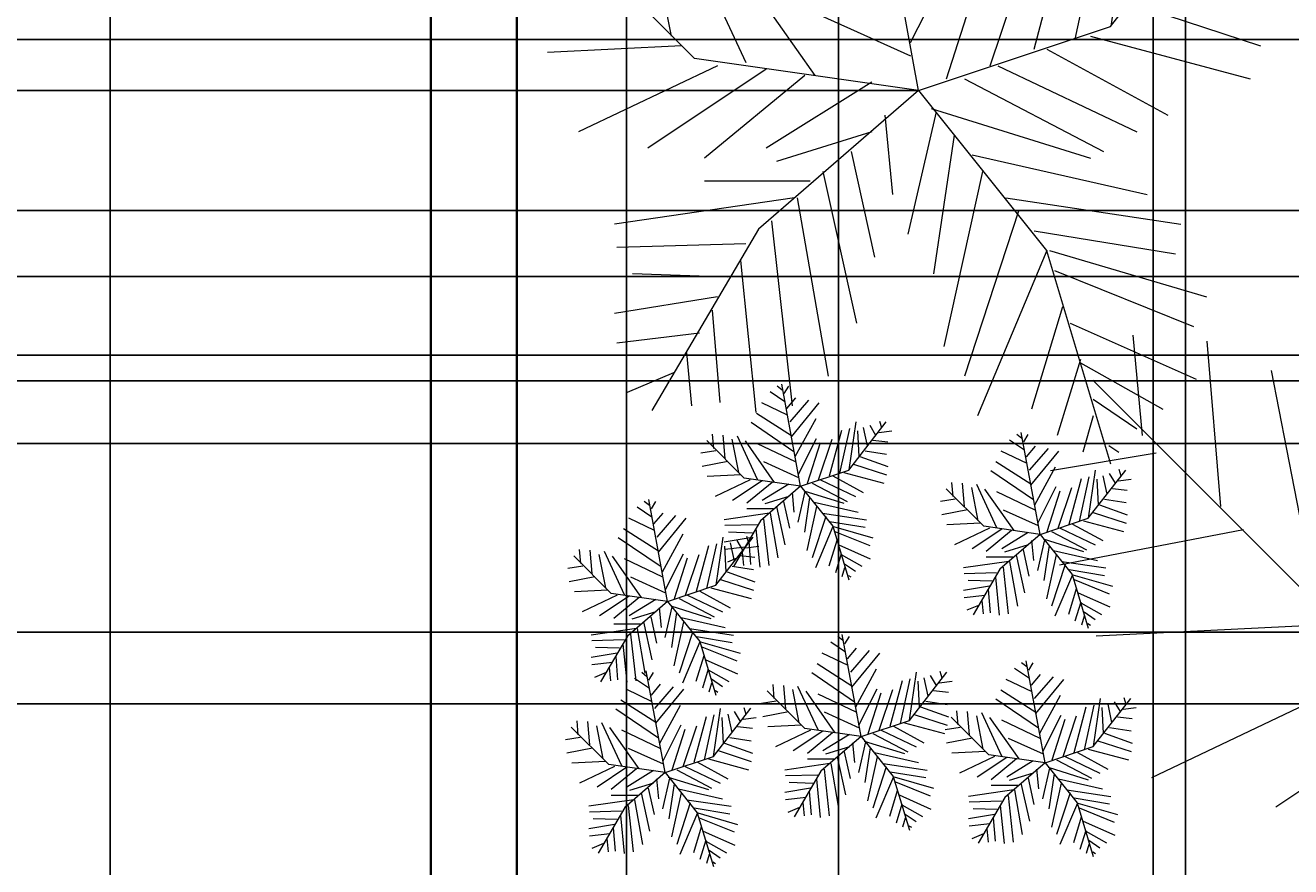
# Model space of a CAD drawing. Units: inches. Extents: x 818 to 1898, y 976 to 2364.
# Tile 59 of 96: x 950 to 1083, y 1958 to 2046. Entities that reach past the tile are written whole.
import ezdxf

# ---------------------------------------------------------------- set-up
doc = ezdxf.new("R2010")
doc.units = ezdxf.units.IN
doc.header["$LTSCALE"] = 5
doc.header["$MEASUREMENT"] = 0
for name, color, linetype, lineweight in [('A-ANNO-DIMS', 2, 'Continuous', 18), ('C-PROP', 7, 'Continuous', 35), ('L-PLNT-BEDS', 94, 'Continuous', 18)]:
    doc.layers.add(name, color=color, linetype=linetype, lineweight=lineweight)
doc.layers.add('L-PLNT', color=116, linetype='Continuous', lineweight=13, true_color=0x136734)
doc.styles.get("Standard").update_dxf_attribs({"font": 'arial.ttf'})
doc.dimstyles.get("Standard").update_dxf_attribs({"dimtxt": 0.18, "dimasz": 0.18, "dimexe": 0.18, "dimexo": 0.0625, "dimgap": 0.09, "dimtad": 0, "dimtih": 1, "dimtoh": 1, "dimdec": 4, "dimzin": 0, "dimdsep": 46, "dimtxsty": 'Standard', "dimcen": 0.09, "dimadec": 0, "dimazin": 0, "dimtfac": 1, "dimtdec": 4, "dimtofl": 0, "dimtmove": 0, "dimatfit": 3, "dimfxl": 1, "dimtolj": 1, "dimtzin": 0, "dimarcsym": 0})

# ---------------------------------------------------------------- blocks, each defined once
blk = doc.blocks.new('SHRUB-ACCENT')
for p, q in [((8.53, 19.84), (7.99, 20.28)), ((10.44, 9.82), (8.47, 20.47)), ((8.74, 19.5), (9.21, 20.28)), ((8.8, 18.63), (7.25, 19.67)), ((9.01, 17.93), (9.96, 19.06)), ((9.35, 16.54), (11.31, 18.8)), ((9.48, 15.07), (5.82, 17.41)), ((9.08, 17.24), (6.37, 18.54)), ((9.48, 14.98), (12.39, 18.54)), ((9.75, 13.42), (5.28, 16.46)), ((9.89, 12.9), (12.06, 16.89)), ((15.49, 11.5), (19.41, 16.55)), ((15.51, 11.51), (16.25, 16.54)), ((17, 15.94), (17.41, 14.03)), ((17.68, 16.2), (18.29, 15.16)), ((18.69, 16.63), (18.9, 15.94)), ((4.55, 10.66), (0.62, 14.58)), ((1.35, 13.77), (1.22, 15.24)), ((2.3, 15.16), (2.51, 12.72)), ((3.25, 14.72), (3.93, 11.25)), ((3.79, 15.07), (5.89, 10.55)), ((10.23, 11.07), (12.12, 14.81)), ((12.33, 10.47), (13.75, 14.72)), ((13.48, 10.9), (14.76, 15.68)), ((14.56, 11.16), (15.58, 15.85)), ((16.39, 15.59), (16.53, 12.9)), ((18.02, 14.63), (19.57, 14.46)), ((18.62, 15.42), (19.98, 15.59)), ((1.56, 13.51), (0, 13.25)), ((7.72, 10.21), (4.67, 14.55)), ((5.89, 14.29), (9.89, 12.38)), ((11.17, 10.12), (12.53, 14.37)), ((17.2, 13.51), (19.44, 13.16)), ((2.84, 12.38), (0.14, 11.86)), ((6.57, 12.38), (10.23, 10.73)), ((15.98, 12.12), (19.44, 10.99)), ((16.66, 12.9), (19.57, 11.86)), ((4.2, 10.99), (0.68, 10.81)), ((10.44, 9.82), (4.55, 10.66)), ((10.44, 9.82), (15.49, 11.5)), ((13.82, 10.9), (17, 9.16)), ((14.97, 11.25), (19.17, 10.12)), ((5.15, 10.47), (1.49, 8.73)), ((6.43, 10.38), (3.32, 8.3)), ((7.45, 10.21), (4.81, 8.04)), ((10.44, 9.82), (6.23, 6.17)), ((9.21, 10.03), (6.43, 8.3)), ((10.44, 9.82), (13.8, 5.61)), ((10.77, 9.34), (14.97, 8.04)), ((11.65, 10.12), (15.31, 8.21)), ((12.53, 10.47), (16.19, 8.73)), ((9.21, 8.73), (6.7, 7.95)), ((8.67, 8.21), (9.28, 5.43)), ((9.55, 9.16), (9.75, 7.08)), ((10.9, 9.25), (10.16, 6.04)), ((11.38, 8.64), (10.84, 5)), ((11.85, 8.12), (16.46, 7.08)), ((7.18, 6.99), (2.44, 6.3)), ((7.59, 7.43), (4.81, 7.43)), ((7.25, 6.99), (8.06, 2.31)), ((7.92, 7.69), (8.8, 3.69)), ((12.12, 7.69), (11.11, 3.09)), ((13.07, 6.65), (11.65, 2.31)), ((12.73, 6.99), (17.34, 6.3)), ((5.89, 5.78), (2.51, 5.69)), ((6.23, 6.17), (3.43, 1.4)), ((5.76, 5.34), (6.16, 1.35)), ((6.57, 6.39), (7.11, 1.52)), ((13.82, 5.6), (11.99, 1.26)), ((13.48, 6.13), (17.2, 5.52)), ((13.8, 5.61), (15.49, 0)), ((13.88, 5.6), (18.02, 4.39)), ((5.15, 4.39), (2.44, 3.95)), ((5.42, 4.91), (2.91, 5)), ((5.01, 4.04), (5.21, 1.61)), ((14.22, 4.13), (13.41, 1.44)), ((14.02, 5.08), (17.68, 3.61)), ((4.67, 3.43), (2.51, 3.17)), ((4.33, 2.91), (4.47, 1.52)), ((14.7, 2.74), (14.09, 0.74)), ((14.43, 3.69), (17.74, 2.22)), ((14.7, 2.65), (16.86, 1.44)), ((4, 2.39), (2.78, 1.87)), ((15.04, 1.7), (16.19, 0.92)), ((15.04, 1.26), (14.76, 0.31)), ((15.44, 0.48), (15.71, 0.31))]:
    blk.add_line(p, q)
blk = doc.blocks.new('PALM-BORDER')
for p, q in [((41.53, 39.05), (33.72, 81.45)), ((33.95, 78.95), (31.8, 80.68)), ((34.76, 77.57), (36.65, 80.68)), ((35.03, 74.11), (28.83, 78.26)), ((35.84, 71.35), (39.61, 75.84)), ((37.18, 65.82), (45, 74.8)), ((36.11, 68.59), (25.33, 73.77)), ((37.72, 59.6), (49.31, 73.77)), ((37.72, 59.95), (23.17, 69.28)), ((39.34, 51.31), (47.96, 67.2)), ((38.8, 53.39), (21.02, 65.48)), ((61.61, 45.75), (77.23, 65.83)), ((61.71, 45.79), (64.67, 65.82)), ((74.37, 66.17), (75.18, 63.4)), ((70.33, 64.44), (72.75, 60.3)), ((53.62, 43.37), (58.74, 62.37)), ((57.93, 44.41), (61.97, 63.06)), ((67.63, 63.4), (69.25, 55.81)), ((65.21, 62.02), (65.75, 51.31)), ((74.1, 61.33), (79.49, 62.02)), ((5.39, 54.77), (4.85, 60.64)), ((9.16, 60.3), (9.97, 50.62)), ((15.09, 59.95), (23.44, 41.99)), ((12.93, 58.57), (15.63, 44.75)), ((40.69, 44.06), (48.23, 58.91)), ((49.04, 41.64), (54.7, 58.57)), ((18.1, 42.4), (2.48, 58.02)), ((30.72, 40.61), (18.59, 57.88)), ((44.46, 40.26), (49.85, 57.19)), ((71.68, 58.22), (77.87, 57.53)), ((23.44, 56.84), (39.34, 49.24)), ((6.2, 53.73), (0, 52.7)), ((68.44, 53.73), (77.33, 52.35)), ((66.29, 51.31), (77.87, 47.17)), ((11.32, 49.24), (0.54, 47.17)), ((26.14, 49.24), (40.69, 42.68)), ((63.59, 48.21), (77.33, 43.71)), ((41.53, 39.05), (61.61, 45.75)), ((16.71, 43.71), (2.69, 43.02)), ((59.55, 44.75), (76.26, 40.26)), ((41.53, 39.05), (18.1, 42.4)), ((54.97, 43.37), (67.63, 36.46)), ((20.48, 41.64), (5.93, 34.73)), ((25.6, 41.3), (13.2, 33.01)), ((49.85, 41.64), (64.4, 34.73)), ((29.64, 40.61), (19.13, 31.97)), ((36.65, 39.91), (25.6, 33.01)), ((46.35, 40.26), (60.9, 32.66)), ((41.53, 39.05), (24.79, 24.55)), ((41.53, 39.05), (54.92, 22.32)), ((42.84, 37.15), (59.55, 31.97)), ((37.99, 36.46), (38.8, 28.17)), ((43.38, 36.81), (40.42, 24.02)), ((36.65, 34.73), (26.68, 31.62)), ((45.27, 34.39), (43.11, 19.88)), ((34.49, 32.66), (36.92, 21.61)), ((47.15, 32.32), (65.48, 28.17)), ((31.53, 30.59), (35.03, 14.7)), ((48.23, 30.59), (44.19, 12.28)), ((30.18, 29.55), (19.13, 29.55)), ((28.56, 27.82), (9.7, 25.06)), ((28.83, 27.82), (32.07, 9.17)), ((50.66, 27.82), (68.98, 25.06)), ((26.14, 25.41), (28.29, 6.06)), ((52, 26.44), (46.35, 9.17)), ((24.79, 24.55), (13.63, 5.58)), ((53.62, 24.37), (68.44, 21.95)), ((23.44, 22.99), (9.97, 22.64)), ((22.9, 21.26), (24.52, 5.37)), ((54.97, 22.3), (47.69, 5.02)), ((54.92, 22.32), (61.61, 0)), ((55.24, 22.3), (71.68, 17.46)), ((21.56, 19.53), (11.59, 19.88)), ((55.78, 20.22), (70.33, 14.35)), ((20.48, 17.46), (9.7, 15.73)), ((19.94, 16.08), (20.75, 6.41)), ((56.59, 16.42), (53.35, 5.72)), ((57.39, 14.7), (70.6, 8.83)), ((18.59, 13.66), (9.97, 12.62)), ((17.24, 11.59), (17.78, 6.06)), ((58.47, 10.9), (56.05, 2.95)), ((15.9, 9.52), (11.05, 7.44)), ((58.47, 10.55), (67.09, 5.72)), ((59.82, 6.75), (64.4, 3.64)), ((59.82, 5.02), (58.74, 1.22)), ((61.44, 1.92), (62.51, 1.22))]:
    blk.add_line(p, q)
blk = doc.blocks.new('PALM-DECK')
for p, q in [((9.63, 97.85), (8.67, 108.34)), ((16.37, 107.72), (17.81, 90.44)), ((23.11, 104.64), (27.92, 79.95)), ((32.33, 75.75), (4.43, 103.66)), ((11.07, 96), (0, 94.15)), ((20.22, 87.97), (0.96, 84.27)), ((29.85, 78.1), (4.81, 76.87)), ((36.59, 74.4), (10.59, 62.05)), ((45.73, 73.78), (23.59, 58.97))]:
    blk.add_line(p, q)
blk = doc.blocks.new('*D59')
at = {"layer": 'A-ANNO-DIMS', "color": 0, "lineweight": -2, "ltscale": 5, "transparency": 16777216}
for p, q in [((1251.64, 2300.39), (818.03, 2300.39)), ((818.21, 2300.21), (818.21, 1669.95)), ((818.21, 1039.32), (818.21, 1669.59)), ((896.05, 1039.14), (818.03, 1039.14))]:
    blk.add_line(p, q, dxfattribs=at)
at = {"layer": 'A-ANNO-DIMS', "color": 0, "ltscale": 5, "transparency": 16777216}
for points in [[(818.18, 2300.21), (818.24, 2300.21), (818.21, 2300.39)], [(818.18, 1039.32), (818.24, 1039.32), (818.21, 1039.14)]]:
    blk.add_solid(points, dxfattribs=at)
at = {"layer": 'Defpoints', "color": 0, "ltscale": 5, "transparency": 16777216}
for p in [(818.21, 2300.39), (1251.71, 2300.39), (896.11, 1039.14)]:
    blk.add_point(p, dxfattribs=at)
at = {"layer": 'A-ANNO-DIMS', "color": 0, "ltscale": 5, "transparency": 16777216, "insert": (818.21, 1669.77), "char_height": 0.18, "attachment_point": 5}
blk.add_mtext('\\A1;1261.2', dxfattribs=at)
blk = doc.blocks.new('*D60')
at = {"layer": 'A-ANNO-DIMS', "color": 0, "lineweight": -2, "ltscale": 5, "transparency": 16777216}
for p, q in [((992.66, 2294.22), (818.03, 2294.22)), ((818.21, 2294.04), (818.21, 1748.77)), ((818.21, 1203.14), (818.21, 1748.41)), ((992.66, 1202.96), (818.03, 1202.96))]:
    blk.add_line(p, q, dxfattribs=at)
at = {"layer": 'A-ANNO-DIMS', "color": 0, "ltscale": 5, "transparency": 16777216}
for points in [[(818.18, 2294.04), (818.24, 2294.04), (818.21, 2294.22)], [(818.18, 1203.14), (818.24, 1203.14), (818.21, 1202.96)]]:
    blk.add_solid(points, dxfattribs=at)
at = {"layer": 'Defpoints', "color": 0, "ltscale": 5, "transparency": 16777216}
for p in [(818.21, 2294.22), (992.73, 2294.22), (992.73, 1202.96)]:
    blk.add_point(p, dxfattribs=at)
at = {"layer": 'A-ANNO-DIMS', "color": 0, "ltscale": 5, "transparency": 16777216, "insert": (818.21, 1748.59), "char_height": 0.18, "attachment_point": 5}
blk.add_mtext('\\A1;1091.3', dxfattribs=at)
blk = doc.blocks.new('*D61')
at = {"layer": 'A-ANNO-DIMS', "color": 0, "lineweight": -2, "ltscale": 5, "transparency": 16777216}
for p, q in [((1071.73, 1203.03), (1071.73, 2363.87)), ((1071.91, 2363.69), (1250.94, 2363.69)), ((1430.55, 2363.69), (1251.51, 2363.69)), ((1430.73, 1203.03), (1430.73, 2363.87))]:
    blk.add_line(p, q, dxfattribs=at)
at = {"layer": 'A-ANNO-DIMS', "color": 0, "ltscale": 5, "transparency": 16777216}
for points in [[(1071.91, 2363.72), (1071.91, 2363.66), (1071.73, 2363.69)], [(1430.55, 2363.72), (1430.55, 2363.66), (1430.73, 2363.69)]]:
    blk.add_solid(points, dxfattribs=at)
at = {"layer": 'Defpoints', "color": 0, "ltscale": 5, "transparency": 16777216}
for p in [(1430.73, 2363.69), (1071.73, 1202.96), (1430.73, 1202.96)]:
    blk.add_point(p, dxfattribs=at)
at = {"layer": 'A-ANNO-DIMS', "color": 0, "ltscale": 5, "transparency": 16777216, "insert": (1251.23, 2363.69), "char_height": 0.18, "attachment_point": 5}
blk.add_mtext('\\A1;359', dxfattribs=at)
blk = doc.blocks.new('*D73')
at = {"layer": 'A-ANNO-DIMS', "color": 0, "lineweight": -2, "ltscale": 5, "transparency": 16777216}
for p, q in [((1590.66, 2011.08), (818.03, 2011.08)), ((818.21, 2010.9), (818.21, 1996.76)), ((818.21, 1982.26), (818.21, 1996.4)), ((1590.66, 1982.08), (818.03, 1982.08))]:
    blk.add_line(p, q, dxfattribs=at)
at = {"layer": 'A-ANNO-DIMS', "color": 0, "ltscale": 5, "transparency": 16777216}
for points in [[(818.18, 2010.9), (818.24, 2010.9), (818.21, 2011.08)], [(818.18, 1982.26), (818.24, 1982.26), (818.21, 1982.08)]]:
    blk.add_solid(points, dxfattribs=at)
at = {"layer": 'Defpoints', "color": 0, "ltscale": 5, "transparency": 16777216}
for p in [(818.21, 2011.08), (1590.73, 2011.08), (1590.73, 1982.08)]:
    blk.add_point(p, dxfattribs=at)
at = {"layer": 'A-ANNO-DIMS', "color": 0, "ltscale": 5, "transparency": 16777216, "insert": (818.21, 1996.58), "char_height": 0.18, "attachment_point": 5}
blk.add_mtext('\\A1;29', dxfattribs=at)
blk = doc.blocks.new('*D79')
at = {"layer": 'A-ANNO-DIMS', "color": 0, "lineweight": -2, "ltscale": 5, "transparency": 16777216}
for p, q in [((992.73, 1203.03), (992.73, 2363.87)), ((992.91, 2363.69), (1032.01, 2363.69)), ((1071.55, 2363.69), (1032.44, 2363.69)), ((1071.73, 1203.03), (1071.73, 2363.87))]:
    blk.add_line(p, q, dxfattribs=at)
at = {"layer": 'A-ANNO-DIMS', "color": 0, "ltscale": 5, "transparency": 16777216}
for points in [[(992.91, 2363.72), (992.91, 2363.66), (992.73, 2363.69)], [(1071.55, 2363.72), (1071.55, 2363.66), (1071.73, 2363.69)]]:
    blk.add_solid(points, dxfattribs=at)
at = {"layer": 'Defpoints', "color": 0, "ltscale": 5, "transparency": 16777216}
for p in [(1071.73, 2363.69), (992.73, 1202.96), (1071.73, 1202.96)]:
    blk.add_point(p, dxfattribs=at)
at = {"layer": 'A-ANNO-DIMS', "color": 0, "ltscale": 5, "transparency": 16777216, "insert": (1032.23, 2363.69), "char_height": 0.18, "attachment_point": 5}
blk.add_mtext('\\A1;79', dxfattribs=at)
blk = doc.blocks.new('*D90')
at = {"layer": 'A-ANNO-DIMS', "color": 0, "lineweight": -2, "ltscale": 5, "transparency": 16777216}
for p, q in [((904.95, 1071.12), (904.95, 2363.87)), ((905.13, 2363.69), (931.67, 2363.69)), ((958.99, 2363.69), (932.45, 2363.69)), ((959.17, 1071.12), (959.17, 2363.87))]:
    blk.add_line(p, q, dxfattribs=at)
at = {"layer": 'A-ANNO-DIMS', "color": 0, "ltscale": 5, "transparency": 16777216}
for points in [[(905.13, 2363.72), (905.13, 2363.66), (904.95, 2363.69)], [(958.99, 2363.72), (958.99, 2363.66), (959.17, 2363.69)]]:
    blk.add_solid(points, dxfattribs=at)
at = {"layer": 'Defpoints', "color": 0, "ltscale": 5, "transparency": 16777216}
for p in [(959.17, 2363.69), (904.95, 1071.06), (959.17, 1071.06)]:
    blk.add_point(p, dxfattribs=at)
at = {"layer": 'A-ANNO-DIMS', "color": 0, "ltscale": 5, "transparency": 16777216, "insert": (932.06, 2363.69), "char_height": 0.18, "attachment_point": 5}
blk.add_mtext('\\A1;54.22', dxfattribs=at)
blk = doc.blocks.new('*D91')
at = {"layer": 'A-ANNO-DIMS', "color": 0, "lineweight": -2, "ltscale": 5, "transparency": 16777216}
for p, q in [((959.17, 1071.12), (959.17, 2363.87)), ((959.35, 2363.69), (985.8, 2363.69)), ((1013.04, 2363.69), (986.59, 2363.69)), ((1013.22, 1071.12), (1013.22, 2363.87))]:
    blk.add_line(p, q, dxfattribs=at)
at = {"layer": 'A-ANNO-DIMS', "color": 0, "ltscale": 5, "transparency": 16777216}
for points in [[(959.35, 2363.72), (959.35, 2363.66), (959.17, 2363.69)], [(1013.04, 2363.72), (1013.04, 2363.66), (1013.22, 2363.69)]]:
    blk.add_solid(points, dxfattribs=at)
at = {"layer": 'Defpoints', "color": 0, "ltscale": 5, "transparency": 16777216}
for p in [(1013.22, 2363.69), (959.17, 1071.06), (1013.22, 1071.06)]:
    blk.add_point(p, dxfattribs=at)
at = {"layer": 'A-ANNO-DIMS', "color": 0, "ltscale": 5, "transparency": 16777216, "insert": (986.2, 2363.69), "char_height": 0.18, "attachment_point": 5}
blk.add_mtext('\\A1;54.04', dxfattribs=at)
blk = doc.blocks.new('*D92')
at = {"layer": 'A-ANNO-DIMS', "color": 0, "lineweight": -2, "ltscale": 5, "transparency": 16777216}
for p, q in [((1013.22, 1071.12), (1013.22, 2363.87)), ((1013.4, 2363.69), (1040.38, 2363.69)), ((1068.16, 2363.69), (1041.17, 2363.69)), ((1068.34, 1071.12), (1068.34, 2363.87))]:
    blk.add_line(p, q, dxfattribs=at)
at = {"layer": 'A-ANNO-DIMS', "color": 0, "ltscale": 5, "transparency": 16777216}
for points in [[(1013.4, 2363.72), (1013.4, 2363.66), (1013.22, 2363.69)], [(1068.16, 2363.72), (1068.16, 2363.66), (1068.34, 2363.69)]]:
    blk.add_solid(points, dxfattribs=at)
at = {"layer": 'Defpoints', "color": 0, "ltscale": 5, "transparency": 16777216}
for p in [(1068.34, 2363.69), (1013.22, 1071.06), (1068.34, 1071.06)]:
    blk.add_point(p, dxfattribs=at)
at = {"layer": 'A-ANNO-DIMS', "color": 0, "ltscale": 5, "transparency": 16777216, "insert": (1040.78, 2363.69), "char_height": 0.18, "attachment_point": 5}
blk.add_mtext('\\A1;55.12', dxfattribs=at)
blk = doc.blocks.new('*D93')
at = {"layer": 'A-ANNO-DIMS', "color": 0, "lineweight": -2, "ltscale": 5, "transparency": 16777216}
for p, q in [((1068.34, 1071.12), (1068.34, 2363.87)), ((1068.52, 2363.69), (1094.16, 2363.69)), ((1120.58, 2363.69), (1094.94, 2363.69)), ((1120.76, 1071.12), (1120.76, 2363.87))]:
    blk.add_line(p, q, dxfattribs=at)
at = {"layer": 'A-ANNO-DIMS', "color": 0, "ltscale": 5, "transparency": 16777216}
for points in [[(1068.52, 2363.72), (1068.52, 2363.66), (1068.34, 2363.69)], [(1120.58, 2363.72), (1120.58, 2363.66), (1120.76, 2363.69)]]:
    blk.add_solid(points, dxfattribs=at)
at = {"layer": 'Defpoints', "color": 0, "ltscale": 5, "transparency": 16777216}
for p in [(1120.76, 2363.69), (1068.34, 1071.06), (1120.76, 1071.06)]:
    blk.add_point(p, dxfattribs=at)
at = {"layer": 'A-ANNO-DIMS', "color": 0, "ltscale": 5, "transparency": 16777216, "insert": (1094.55, 2363.69), "char_height": 0.18, "attachment_point": 5}
blk.add_mtext('\\A1;52.42', dxfattribs=at)
blk = doc.blocks.new('*D124')
at = {"layer": 'A-ANNO-DIMS', "color": 0, "lineweight": -2, "ltscale": 5, "transparency": 16777216}
for p, q in [((1131.7, 1974.57), (818.03, 1974.57)), ((818.21, 1974.39), (818.21, 1884.68)), ((818.21, 1794.61), (818.21, 1884.32)), ((1138.44, 1794.43), (818.03, 1794.43))]:
    blk.add_line(p, q, dxfattribs=at)
at = {"layer": 'A-ANNO-DIMS', "color": 0, "ltscale": 5, "transparency": 16777216}
for points in [[(818.18, 1974.39), (818.24, 1974.39), (818.21, 1974.57)], [(818.18, 1794.61), (818.24, 1794.61), (818.21, 1794.43)]]:
    blk.add_solid(points, dxfattribs=at)
at = {"layer": 'Defpoints', "color": 0, "ltscale": 5, "transparency": 16777216}
for p in [(818.21, 1974.57), (1131.77, 1974.57), (1138.5, 1794.43)]:
    blk.add_point(p, dxfattribs=at)
at = {"layer": 'A-ANNO-DIMS', "color": 0, "ltscale": 5, "transparency": 16777216, "insert": (818.21, 1884.5), "char_height": 0.18, "attachment_point": 5}
blk.add_mtext('\\A1;180.14', dxfattribs=at)
blk = doc.blocks.new('*D125')
at = {"layer": 'A-ANNO-DIMS', "color": 0, "lineweight": -2, "ltscale": 5, "transparency": 16777216}
for p, q in [((1083.66, 2044.08), (818.03, 2044.08)), ((818.21, 2043.9), (818.21, 2009.51)), ((818.21, 1974.75), (818.21, 2009.14)), ((1131.7, 1974.57), (818.03, 1974.57))]:
    blk.add_line(p, q, dxfattribs=at)
at = {"layer": 'A-ANNO-DIMS', "color": 0, "ltscale": 5, "transparency": 16777216}
for points in [[(818.18, 2043.9), (818.24, 2043.9), (818.21, 2044.08)], [(818.18, 1974.75), (818.24, 1974.75), (818.21, 1974.57)]]:
    blk.add_solid(points, dxfattribs=at)
at = {"layer": 'Defpoints', "color": 0, "ltscale": 5, "transparency": 16777216}
for p in [(1083.73, 2044.08), (818.21, 1974.57), (1131.77, 1974.57)]:
    blk.add_point(p, dxfattribs=at)
at = {"layer": 'A-ANNO-DIMS', "color": 0, "ltscale": 5, "transparency": 16777216, "insert": (818.21, 2009.33), "char_height": 0.18, "attachment_point": 5}
blk.add_mtext('\\A1;69.5', dxfattribs=at)
blk = doc.blocks.new('*D126')
at = {"layer": 'A-ANNO-DIMS', "color": 0, "lineweight": -2, "ltscale": 5, "transparency": 16777216}
for p, q in [((1035.38, 1252.09), (1035.38, 2363.87)), ((1035.56, 2363.69), (1075.41, 2363.69)), ((1116.01, 2363.69), (1076.16, 2363.69)), ((1116.19, 1236.03), (1116.19, 2363.87))]:
    blk.add_line(p, q, dxfattribs=at)
at = {"layer": 'A-ANNO-DIMS', "color": 0, "ltscale": 5, "transparency": 16777216}
for points in [[(1035.56, 2363.72), (1035.56, 2363.66), (1035.38, 2363.69)], [(1116.01, 2363.72), (1116.01, 2363.66), (1116.19, 2363.69)]]:
    blk.add_solid(points, dxfattribs=at)
at = {"layer": 'Defpoints', "color": 0, "ltscale": 5, "transparency": 16777216}
for p in [(1035.38, 2363.69), (1035.38, 1252.02), (1116.19, 1235.96)]:
    blk.add_point(p, dxfattribs=at)
at = {"layer": 'A-ANNO-DIMS', "color": 0, "ltscale": 5, "transparency": 16777216, "insert": (1075.78, 2363.69), "char_height": 0.18, "attachment_point": 5}
blk.add_mtext('\\A1;80.81', dxfattribs=at)
blk = doc.blocks.new('*D132')
at = {"layer": 'A-ANNO-DIMS', "color": 0, "lineweight": -2, "ltscale": 5, "transparency": 16777216}
for p, q in [((1043.71, 2038.76), (818.03, 2038.76)), ((818.21, 2038.58), (818.21, 1963.01)), ((818.21, 1887.08), (818.21, 1962.65)), ((1043.71, 1886.9), (818.03, 1886.9))]:
    blk.add_line(p, q, dxfattribs=at)
at = {"layer": 'A-ANNO-DIMS', "color": 0, "ltscale": 5, "transparency": 16777216}
for points in [[(818.18, 2038.58), (818.24, 2038.58), (818.21, 2038.76)], [(818.18, 1887.08), (818.24, 1887.08), (818.21, 1886.9)]]:
    blk.add_solid(points, dxfattribs=at)
at = {"layer": 'Defpoints', "color": 0, "ltscale": 5, "transparency": 16777216}
for p in [(818.21, 2038.76), (1043.77, 2038.76), (1043.77, 1886.9)]:
    blk.add_point(p, dxfattribs=at)
at = {"layer": 'A-ANNO-DIMS', "color": 0, "ltscale": 5, "transparency": 16777216, "insert": (818.21, 1962.83), "char_height": 0.18, "attachment_point": 5}
blk.add_mtext('\\A1;151.86', dxfattribs=at)
blk = doc.blocks.new('*D133')
at = {"layer": 'A-ANNO-DIMS', "color": 0, "lineweight": -2, "ltscale": 5, "transparency": 16777216}
for p, q in [((1041.64, 2162.89), (818.03, 2162.89)), ((818.21, 2162.71), (818.21, 2101.01)), ((818.21, 2038.94), (818.21, 2100.64)), ((1043.71, 2038.76), (818.03, 2038.76))]:
    blk.add_line(p, q, dxfattribs=at)
at = {"layer": 'A-ANNO-DIMS', "color": 0, "ltscale": 5, "transparency": 16777216}
for points in [[(818.18, 2162.71), (818.24, 2162.71), (818.21, 2162.89)], [(818.18, 2038.94), (818.24, 2038.94), (818.21, 2038.76)]]:
    blk.add_solid(points, dxfattribs=at)
at = {"layer": 'Defpoints', "color": 0, "ltscale": 5, "transparency": 16777216}
for p in [(818.21, 2162.89), (1041.7, 2162.89), (1043.77, 2038.76)]:
    blk.add_point(p, dxfattribs=at)
at = {"layer": 'A-ANNO-DIMS', "color": 0, "ltscale": 5, "transparency": 16777216, "insert": (818.21, 2100.82), "char_height": 0.18, "attachment_point": 5}
blk.add_mtext('\\A1;124.13', dxfattribs=at)
blk = doc.blocks.new('*D207')
at = {"layer": 'A-ANNO-DIMS', "color": 0, "lineweight": -2, "ltscale": 5, "transparency": 16777216}
for p, q in [((1590.66, 2044.08), (818.03, 2044.08)), ((818.21, 2043.9), (818.21, 2027.76)), ((818.21, 2011.26), (818.21, 2027.4)), ((1590.66, 2011.08), (818.03, 2011.08))]:
    blk.add_line(p, q, dxfattribs=at)
at = {"layer": 'A-ANNO-DIMS', "color": 0, "ltscale": 5, "transparency": 16777216}
for points in [[(818.18, 2043.9), (818.24, 2043.9), (818.21, 2044.08)], [(818.18, 2011.26), (818.24, 2011.26), (818.21, 2011.08)]]:
    blk.add_solid(points, dxfattribs=at)
at = {"layer": 'Defpoints', "color": 0, "ltscale": 5, "transparency": 16777216}
for p in [(818.21, 2044.08), (1590.73, 2044.08), (1590.73, 2011.08)]:
    blk.add_point(p, dxfattribs=at)
at = {"layer": 'A-ANNO-DIMS', "color": 0, "ltscale": 5, "transparency": 16777216, "insert": (818.21, 2027.58), "char_height": 0.18, "attachment_point": 5}
blk.add_mtext('\\A1;33', dxfattribs=at)
blk = doc.blocks.new('*D232')
at = {"layer": 'A-ANNO-DIMS', "color": 0, "lineweight": -2, "ltscale": 5, "transparency": 16777216}
for p, q in [((1303.87, 2008.39), (818.03, 2008.39)), ((818.21, 2008.21), (818.21, 1980.9)), ((818.21, 1953.22), (818.21, 1980.53)), ((1303.87, 1953.04), (818.03, 1953.04))]:
    blk.add_line(p, q, dxfattribs=at)
at = {"layer": 'A-ANNO-DIMS', "color": 0, "ltscale": 5, "transparency": 16777216}
for points in [[(818.18, 2008.21), (818.24, 2008.21), (818.21, 2008.39)], [(818.18, 1953.22), (818.24, 1953.22), (818.21, 1953.04)]]:
    blk.add_solid(points, dxfattribs=at)
at = {"layer": 'Defpoints', "color": 0, "ltscale": 5, "transparency": 16777216}
for p in [(818.21, 2008.39), (1303.93, 2008.39), (1303.93, 1953.04)]:
    blk.add_point(p, dxfattribs=at)
at = {"layer": 'A-ANNO-DIMS', "color": 0, "ltscale": 5, "transparency": 16777216, "insert": (818.21, 1980.72), "char_height": 0.18, "attachment_point": 5}
blk.add_mtext('\\A1;55.35', dxfattribs=at)
blk = doc.blocks.new('*D234')
at = {"layer": 'A-ANNO-DIMS', "color": 0, "lineweight": -2, "ltscale": 5, "transparency": 16777216}
for p, q in [((1267.66, 2044.08), (818.03, 2044.08)), ((818.21, 2043.9), (818.21, 2026.42)), ((818.21, 2008.57), (818.21, 2026.05)), ((1303.87, 2008.39), (818.03, 2008.39))]:
    blk.add_line(p, q, dxfattribs=at)
at = {"layer": 'A-ANNO-DIMS', "color": 0, "ltscale": 5, "transparency": 16777216}
for points in [[(818.18, 2043.9), (818.24, 2043.9), (818.21, 2044.08)], [(818.18, 2008.57), (818.24, 2008.57), (818.21, 2008.39)]]:
    blk.add_solid(points, dxfattribs=at)
at = {"layer": 'Defpoints', "color": 0, "ltscale": 5, "transparency": 16777216}
for p in [(818.21, 2044.08), (1267.73, 2044.08), (1303.93, 2008.39)]:
    blk.add_point(p, dxfattribs=at)
at = {"layer": 'A-ANNO-DIMS', "color": 0, "ltscale": 5, "transparency": 16777216, "insert": (818.21, 2026.23), "char_height": 0.18, "attachment_point": 5}
blk.add_mtext('\\A1;35.69', dxfattribs=at)
blk = doc.blocks.new('*D237')
at = {"layer": 'A-ANNO-DIMS', "color": 0, "lineweight": -2, "ltscale": 5, "transparency": 16777216}
for p, q in [((1310.85, 2026.21), (818.03, 2026.21)), ((818.21, 2026.03), (818.21, 2014.2)), ((818.21, 2002), (818.21, 2013.83)), ((1314.2, 2001.82), (818.03, 2001.82))]:
    blk.add_line(p, q, dxfattribs=at)
at = {"layer": 'A-ANNO-DIMS', "color": 0, "ltscale": 5, "transparency": 16777216}
for points in [[(818.18, 2026.03), (818.24, 2026.03), (818.21, 2026.21)], [(818.18, 2002), (818.24, 2002), (818.21, 2001.82)]]:
    blk.add_solid(points, dxfattribs=at)
at = {"layer": 'Defpoints', "color": 0, "ltscale": 5, "transparency": 16777216}
for p in [(1310.91, 2026.21), (818.21, 2001.82), (1314.26, 2001.82)]:
    blk.add_point(p, dxfattribs=at)
at = {"layer": 'A-ANNO-DIMS', "color": 0, "ltscale": 5, "transparency": 16777216, "insert": (818.21, 2014.02), "char_height": 0.18, "attachment_point": 5}
blk.add_mtext('\\A1;24.383', dxfattribs=at)
blk = doc.blocks.new('*D248')
at = {"layer": 'A-ANNO-DIMS', "color": 0, "lineweight": -2, "ltscale": 5, "transparency": 16777216}
for p, q in [((1258.66, 2019.29), (818.03, 2019.29)), ((818.21, 2019.11), (818.21, 1974.29)), ((818.21, 1929.1), (818.21, 1973.92)), ((1258.66, 1928.92), (818.03, 1928.92))]:
    blk.add_line(p, q, dxfattribs=at)
at = {"layer": 'A-ANNO-DIMS', "color": 0, "ltscale": 5, "transparency": 16777216}
for points in [[(818.18, 2019.11), (818.24, 2019.11), (818.21, 2019.29)], [(818.18, 1929.1), (818.24, 1929.1), (818.21, 1928.92)]]:
    blk.add_solid(points, dxfattribs=at)
at = {"layer": 'Defpoints', "color": 0, "ltscale": 5, "transparency": 16777216}
for p in [(818.21, 2019.29), (1258.73, 2019.29), (1258.73, 1928.92)]:
    blk.add_point(p, dxfattribs=at)
at = {"layer": 'A-ANNO-DIMS', "color": 0, "ltscale": 5, "transparency": 16777216, "insert": (818.21, 1974.1), "char_height": 0.18, "attachment_point": 5}
blk.add_mtext('\\A1;90.37', dxfattribs=at)

msp = doc.modelspace()

# ---------------------------------------------------------------- linework, layer by layer
at = {"layer": 'C-PROP'}
for p, q in [((992.7251, 2294.2171), (992.7251, 1202.9642)), ((1001.7252, 2285.2171), (1001.7252, 1211.9642))]:
    msp.add_line(p, q, dxfattribs=at)
at = {"layer": 'L-PLNT-BEDS'}
msp.add_line((1071.7251, 2214.9709), (1071.7251, 1202.9642), dxfattribs=at)

# ---------------------------------------------------------------- block references
at = {"layer": 'L-PLNT'}
for name, p in [('PALM-BORDER', (1002.2407, 1999.7071)), ('PALM-DECK', (1057.571, 1904.8049)), ('SHRUB-ACCENT', (1020.9869, 1987.5452)), ('SHRUB-ACCENT', (1046.0558, 1982.4944)), ('SHRUB-ACCENT', (1007.0683, 1975.4824)), ('SHRUB-ACCENT', (1027.3267, 1961.3515)), ('SHRUB-ACCENT', (1046.5756, 1958.6017)), ('SHRUB-ACCENT', (1006.8083, 1957.5628))]:
    msp.add_blockref(name, p, dxfattribs=at)

# ---------------------------------------------------------------- dimensions: what is measured, and where the dimension line sits
at = {"layer": 'A-ANNO-DIMS', "ltscale": 5}
for base, p1, p2, override, picture, middle in [((959.1737, 2363.6929), (904.9504, 1071.0552), (959.1737, 1071.0552), {"dimdec": 2, "dimlfac": 1, "dimrnd": 0, "dimzin": 0, "dimdsep": 46, "dimlunit": 2}, '*D90', (932.062, 2363.6929)), ((1013.2176, 2363.6929), (959.1737, 1071.0552), (1013.2176, 1071.0552), {"dimdec": 2, "dimlfac": 1, "dimrnd": 0, "dimzin": 0, "dimdsep": 46, "dimlunit": 2}, '*D91', (986.1956, 2363.6929)), ((1071.7251, 2363.6929), (992.7251, 1202.9642), (1071.7251, 1202.9642), {"dimdec": 0, "dimlfac": 1, "dimrnd": 0, "dimzin": 0, "dimdsep": 46, "dimlunit": 2}, '*D79', (1032.2251, 2363.6929)), ((1068.3377, 2363.6929), (1013.2176, 1071.0552), (1068.3377, 1071.0552), {"dimdec": 2, "dimlfac": 1, "dimrnd": 0, "dimzin": 0, "dimdsep": 46, "dimlunit": 2}, '*D92', (1040.7776, 2363.6929)), ((1035.3768, 2363.6929), (1116.1882, 1235.9642), (1035.3768, 1252.0242), {"dimdec": 2, "dimlfac": 1, "dimrnd": 0, "dimzin": 0, "dimdsep": 46, "dimlunit": 2}, '*D126', (1075.7825, 2363.6929)), ((1120.7618, 2363.6929), (1068.3377, 1071.0552), (1120.7618, 1071.0552), {"dimdec": 2, "dimlfac": 1, "dimrnd": 0, "dimzin": 0, "dimdsep": 46, "dimlunit": 2}, '*D93', (1094.5497, 2363.6929)), ((1430.7251, 2363.6929), (1071.7251, 1202.9642), (1430.7251, 1202.9642), {"dimdec": 0, "dimlfac": 1, "dimrnd": 0, "dimzin": 0, "dimdsep": 46, "dimlunit": 2}, '*D61', (1251.2251, 2363.6929))]:
    dim = msp.add_linear_dim(base=base, p1=p1, p2=p2, dimstyle='Standard', override=override, dxfattribs=at)
    dim.commit()
    dim.dimension.update_dxf_attribs({"geometry": picture, "text_midpoint": middle})
for base, p1, p2, override, picture, middle in [((818.2059, 2300.3929), (896.1138, 1039.1433), (1251.7057, 2300.3929), {"dimdec": 1, "dimlfac": 1, "dimrnd": 0, "dimzin": 0, "dimdsep": 46, "dimlunit": 2}, '*D59', (818.2059, 1669.7681)), ((818.2059, 2294.2171), (992.7251, 1202.9642), (992.7251, 2294.2171), {"dimdec": 1, "dimlfac": 1, "dimrnd": 0, "dimzin": 0, "dimdsep": 46, "dimlunit": 2}, '*D60', (818.2059, 1748.5907)), ((818.2059, 2162.8898), (1043.7685, 2038.7583), (1041.7008, 2162.8898), {"dimdec": 2, "dimlfac": 1, "dimrnd": 0, "dimzin": 0, "dimdsep": 46, "dimlunit": 2}, '*D133', (818.2059, 2100.824)), ((818.2059, 2044.0782), (1303.9314, 2008.3917), (1267.7251, 2044.0782), {"dimdec": 2, "dimlfac": 1, "dimrnd": 0, "dimzin": 0, "dimdsep": 46, "dimlunit": 2}, '*D234', (818.2059, 2026.235)), ((818.2059, 1974.5735), (1083.7251, 2044.0782), (1131.7651, 1974.5735), {"dimdec": 1, "dimlfac": 1, "dimrnd": 0, "dimzin": 0, "dimdsep": 46, "dimlunit": 2}, '*D125', (818.2059, 2009.3258)), ((818.2059, 2044.0782), (1590.7251, 2011.0782), (1590.7251, 2044.0782), {"dimdec": 0, "dimlfac": 1, "dimrnd": 0, "dimzin": 0, "dimdsep": 46, "dimlunit": 2}, '*D207', (818.2059, 2027.5782)), ((818.2059, 2038.7583), (1043.7685, 1886.9018), (1043.7685, 2038.7583), {"dimdec": 2, "dimlfac": 1, "dimrnd": 0, "dimzin": 0, "dimdsep": 46, "dimlunit": 2}, '*D132', (818.2059, 1962.83)), ((818.2059, 2001.8247), (1310.9077, 2026.2074), (1314.2595, 2001.8247), {"dimdec": 3, "dimlfac": 1, "dimrnd": 0, "dimzin": 0, "dimdsep": 46, "dimlunit": 2}, '*D237', (818.2059, 2014.016)), ((818.2059, 2019.2871), (1258.7251, 1928.9218), (1258.7251, 2019.2871), {"dimdec": 2, "dimlfac": 1, "dimrnd": 0, "dimzin": 0, "dimdsep": 46, "dimlunit": 2}, '*D248', (818.2059, 1974.1044)), ((818.2059, 2011.0782), (1590.7251, 1982.0782), (1590.7251, 2011.0782), {"dimdec": 0, "dimlfac": 1, "dimrnd": 0, "dimzin": 0, "dimdsep": 46, "dimlunit": 2}, '*D73', (818.2059, 1996.5782)), ((818.2059, 2008.3917), (1303.9314, 1953.0408), (1303.9314, 2008.3917), {"dimdec": 2, "dimlfac": 1, "dimrnd": 0, "dimzin": 0, "dimdsep": 46, "dimlunit": 2}, '*D232', (818.2059, 1980.7163)), ((818.2059, 1974.5735), (1138.5041, 1794.4325), (1131.7651, 1974.5735), {"dimdec": 2, "dimlfac": 1, "dimrnd": 0, "dimzin": 0, "dimdsep": 46, "dimlunit": 2}, '*D124', (818.2059, 1884.503))]:
    dim = msp.add_linear_dim(base=base, p1=p1, p2=p2, angle=90, dimstyle='Standard', override=override, dxfattribs=at)
    dim.commit()
    dim.dimension.update_dxf_attribs({"geometry": picture, "text_midpoint": middle})

doc.saveas('drawing.dxf')
